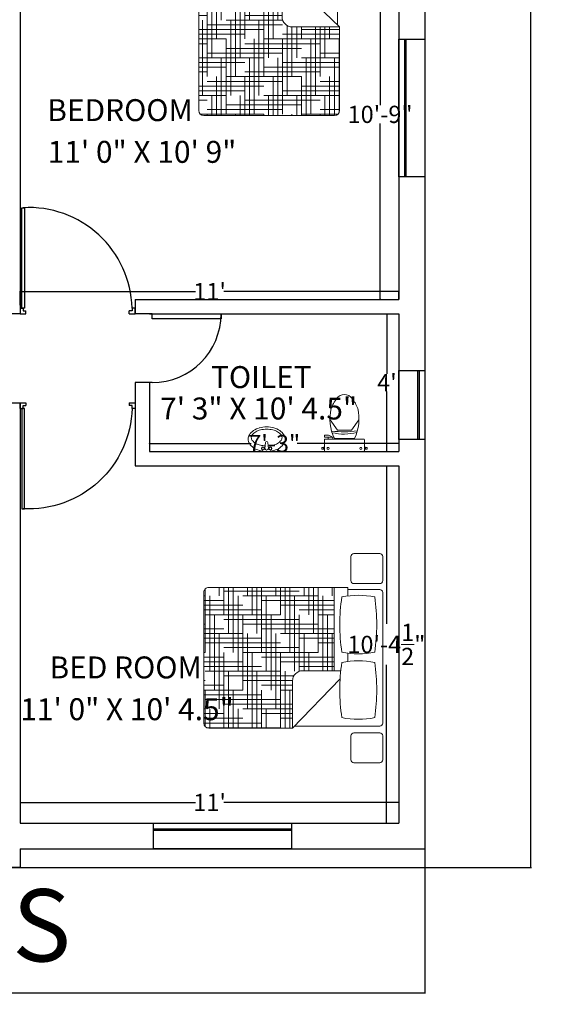
# Model space of a CAD drawing. Units: inches. Extents: x -113 to 5399, y -1393 to 3302.
# Tile 14 of 40: x 1896 to 2086, y 82 to 426. Entities that reach past the tile are written whole.
import ezdxf

# ---------------------------------------------------------------- set-up
doc = ezdxf.new("R2010")
doc.units = ezdxf.units.IN
doc.header["$MEASUREMENT"] = 0
for name, color, linetype, lineweight in [('A-ANNO-DIMS', 254, 'Continuous', 18), ('A-ANNO-TEXT', 7, 'Continuous', 25), ('A-AREA-IDEN', 4, 'Continuous', 18), ('A-FLOR-FIXT', 8, 'Continuous', 18), ('doors', 2, 'Continuous', 25), ('furniture', 131, 'Continuous', 18), ('walls', 1, 'Continuous', 25), ('windows', 3, 'Continuous', 25)]:
    doc.layers.add(name, color=color, linetype=linetype, lineweight=lineweight)
doc.layers.add('A-GLAZ-PATT', color=85, linetype='Continuous', lineweight=13, true_color=0x58ba48)
doc.styles.get("Standard").update_dxf_attribs({"font": 'arial.ttf'})
doc.dimstyles.get("Standard").update_dxf_attribs({"dimtxt": 6, "dimasz": 0.18, "dimexe": 0.18, "dimexo": 0.0625, "dimgap": 0.09, "dimtad": 0, "dimtih": 1, "dimtoh": 1, "dimdec": 1, "dimzin": 0, "dimdsep": 46, "dimlunit": 4, "dimtxsty": 'Standard', "dimblk": 'ARCHTICK', "dimcen": 0.09, "dimadec": 0, "dimazin": 0, "dimtfac": 1, "dimtdec": 1, "dimtofl": 0, "dimtmove": 0, "dimatfit": 3, "dimfxl": 1, "dimtolj": 1, "dimtzin": 0, "dimarcsym": 0})

# ---------------------------------------------------------------- blocks, each defined once
blk = doc.blocks.new('*U2')
for p, q in [((0, 0), (0, -6)), ((24, 0), (24, -6))]:
    blk.add_line(p, q)
blk.add_lwpolyline([(0, 0), (0, 24), (1.75, 24), (1.75, 0)], close=True)
blk.add_arc((0, 0), 24, 0, 90)
blk = doc.blocks.new('*X4')
at = {"color": 0}
for p, q in [((4.3594, 18.5625), (4.3594, 18.6457)), ((4.5, 18), (4.5, 18.6457)), ((4.5469, 18.1875), (4.5469, 18.6457)), ((4.5938, 18.375), (4.5938, 18.6457)), ((4.6406, 18.5625), (4.6406, 18.6457)), ((4.7812, 18), (4.7812, 18.6457)), ((4.8281, 18.1875), (4.8281, 18.6457)), ((4.875, 18.375), (4.875, 18.6457)), ((4.9219, 18.5625), (4.9219, 18.6457)), ((5.0625, 18), (5.0625, 18.6457)), ((5.1094, 18.1875), (5.1094, 18.6457)), ((5.1562, 18.375), (5.1562, 18.6457)), ((5.2031, 18.5625), (5.2031, 18.6457)), ((5.3438, 18), (5.3438, 18.6457)), ((5.3906, 18.1875), (5.3906, 18.6457)), ((5.4375, 18.375), (5.4375, 18.6457)), ((5.4844, 18.5625), (5.4844, 18.6457)), ((5.625, 18), (5.625, 18.6287)), ((4.4531, 17.8169), (4.4531, 18.5625)), ((4.5, 18.5625), (5.25, 18.5625)), ((4.6875, 18.6094), (5.4375, 18.6094)), ((4.7344, 17.8125), (4.7344, 18.5625)), ((5.0156, 17.8125), (5.0156, 18.5625)), ((5.2969, 17.8125), (5.2969, 18.5625)), ((5.5781, 17.8125), (5.5781, 18.5625)), ((5.625, 18.5625), (5.6375, 18.5625)), ((4.3395, 18.5156), (5.0625, 18.5156)), ((4.3395, 18.4688), (4.875, 18.4688)), ((5.25, 18.4688), (5.6375, 18.4688)), ((5.4375, 18.5156), (5.6375, 18.5156)), ((4.3395, 18.4219), (4.6875, 18.4219)), ((4.3395, 18.375), (4.5, 18.375)), ((4.4062, 17.8169), (4.4062, 18.375)), ((4.6875, 17.8114), (4.6875, 18.375)), ((4.6875, 18.3281), (5.4375, 18.3281)), ((4.875, 18.375), (5.625, 18.375)), ((4.9688, 17.625), (4.9688, 18.375)), ((5.0625, 18.4219), (5.6375, 18.4219)), ((5.25, 17.625), (5.25, 18.375)), ((5.5312, 17.625), (5.5312, 18.375)), ((4.3395, 18.2344), (5.0625, 18.2344)), ((4.5, 18.2812), (5.25, 18.2812)), ((5.4375, 18.2344), (5.6375, 18.2344)), ((5.625, 18.2812), (5.6375, 18.2812)), ((4.3395, 18.1875), (4.875, 18.1875)), ((4.3395, 18.1406), (4.6875, 18.1406)), ((4.3594, 17.8169), (4.3594, 18.1875)), ((4.6406, 17.8169), (4.6406, 18.1875)), ((4.9219, 17.4375), (4.9219, 18.1875)), ((5.0625, 18.1406), (5.6375, 18.1406)), ((5.2031, 17.4375), (5.2031, 18.1875)), ((5.25, 18.1875), (5.6375, 18.1875)), ((5.4844, 17.4375), (5.4844, 18.1875)), ((4.3395, 18.0938), (4.5, 18.0938)), ((4.6875, 18.0469), (5.4375, 18.0469)), ((4.875, 18.0938), (5.625, 18.0938)), ((4.3395, 17.9531), (5.0625, 17.9531)), ((4.5, 18), (5.25, 18)), ((4.5938, 17.8169), (4.5938, 18)), ((4.875, 17.25), (4.875, 18)), ((5.1562, 17.25), (5.1562, 18)), ((5.4375, 17.25), (5.4375, 18)), ((5.4375, 17.9531), (5.6375, 17.9531)), ((5.625, 18), (5.6375, 18)), ((4.3395, 17.9062), (4.875, 17.9062)), ((4.3395, 17.8594), (4.6875, 17.8594)), ((5.0625, 17.8594), (5.6375, 17.8594)), ((5.25, 17.9062), (5.6375, 17.9062)), ((4.7421, 17.7656), (5.4375, 17.7656)), ((4.8281, 17.2457), (4.8281, 17.8125)), ((4.875, 17.8125), (5.625, 17.8125)), ((5.1094, 17.2457), (5.1094, 17.8125)), ((5.3906, 17.2457), (5.3906, 17.8125)), ((4.7548, 17.7188), (5.25, 17.7188)), ((4.7548, 17.6719), (5.0625, 17.6719)), ((5.4375, 17.6719), (5.6375, 17.6719)), ((5.625, 17.7188), (5.6375, 17.7188)), ((4.7548, 17.625), (4.875, 17.625)), ((4.7812, 17.2457), (4.7812, 17.625)), ((5.0625, 17.2457), (5.0625, 17.625)), ((5.0625, 17.5781), (5.6375, 17.5781)), ((5.25, 17.625), (5.6375, 17.625)), ((5.3438, 17.2457), (5.3438, 17.625)), ((5.625, 17.2627), (5.625, 17.625)), ((4.7548, 17.4844), (5.4375, 17.4844)), ((4.875, 17.5312), (5.625, 17.5312)), ((4.7548, 17.4375), (5.25, 17.4375)), ((4.7548, 17.3906), (5.0625, 17.3906)), ((5.0156, 17.2457), (5.0156, 17.4375)), ((5.2969, 17.2457), (5.2969, 17.4375)), ((5.4375, 17.3906), (5.6375, 17.3906)), ((5.5781, 17.2457), (5.5781, 17.4375)), ((5.625, 17.4375), (5.6375, 17.4375)), ((4.7548, 17.3438), (4.875, 17.3438)), ((4.875, 17.25), (5.6077, 17.25)), ((4.9688, 17.2457), (4.9688, 17.25)), ((5.0625, 17.2969), (5.6375, 17.2969)), ((5.25, 17.3438), (5.6375, 17.3438)), ((5.25, 17.2457), (5.25, 17.25)), ((5.5312, 17.2457), (5.5312, 17.25))]:
    blk.add_line(p, q, dxfattribs=at)
blk = doc.blocks.new('MAT-P01')
for p, q in [((-0.0213, 0.8164), (-0.0213, 0.5605)), ((0.0087, 0.8464), (0.2471, 0.8464)), ((0.2771, 0.8164), (0.2771, 0.5605)), ((0.3437, 0.8164), (0.3437, -0.0316)), ((0.3737, 0.8464), (1.6737, 0.8464)), ((1.7037, 0.8164), (1.7037, 0.5005)), ((1.7622, 0.8164), (1.7622, 0.5605)), ((1.7922, 0.8464), (2.0306, 0.8464)), ((2.0606, 0.8164), (2.0606, 0.5605)), ((0.0087, 0.5305), (0.2471, 0.5305)), ((0.9879, 0.5005), (1.0693, 0.5005)), ((1.6393, 0.5005), (1.7237, 0.5005)), ((1.7237, 0.5005), (1.7237, -0.8836)), ((1.7922, 0.5305), (2.0306, 0.5305)), ((0.8146, 0.423), (0.3237, -0.0509)), ((0.8949, 0.4293), (0.8949, 0.0491)), ((0.8949, 0.3643), (1.7237, 0.3643)), ((0.8949, 0.3643), (0.8949, 0.0491)), ((0.8949, 0.3643), (1.7237, 0.3643)), ((1.7237, 0.3643), (1.7237, -0.8836)), ((0.3237, -0.0509), (0.7949, -0.0509)), ((0.3237, -0.0509), (0.3237, -0.8836)), ((0.3737, -0.9336), (1.6737, -0.9336))]:
    blk.add_line(p, q)
for centre, radius, start, end in [((0.0087, 0.8164), 0.03, 90, 180), ((0.2471, 0.8164), 0.03, 0, 90), ((0.3737, 0.8164), 0.03, 90, 180), ((0.7029, -1.1436), 1.9306, 81.81622, 98.18378), ((1.3543, -1.1436), 1.9306, 81.81622, 98.18378), ((1.6737, 0.8164), 0.03, 0, 90), ((1.7922, 0.8164), 0.03, 90, 180), ((2.0306, 0.8164), 0.03, 0, 90), ((1.2251, 0.6034), 0.8138, 168.37298, 191.62702), ((0.1806, 0.6034), 0.8138, 348.37298, 11.62702), ((1.8766, 0.6034), 0.8138, 168.37298, 191.62702), ((0.8321, 0.6034), 0.8138, 348.37298, 11.62702), ((0.0087, 0.5605), 0.03, 180, 270), ((0.2471, 0.5605), 0.03, 270, 0), ((1.7922, 0.5605), 0.03, 180, 270), ((2.0306, 0.5605), 0.03, 270, 0), ((0.7029, 2.3504), 1.9306, 261.81622, 278.18378), ((1.3543, 2.3504), 1.9306, 261.81622, 278.18378), ((0.7949, 0.0491), 0.1, 270, 0), ((0.3737, -0.8836), 0.05, 180, 270), ((1.6737, -0.8836), 0.05, 270, 0)]:
    blk.add_arc(centre, radius, start, end)
at = {"rotation": 270}
blk.add_blockref('*X4', (-16.9221, 4.7038), dxfattribs=at)
blk = doc.blocks.new('toilet-3')
at = {"color": 0, "linetype": 'ByBlock'}
for p, q in [((-0.281, -0.05), (-0.281, -0.069)), ((-0.281, -0.05), (-0.261, -0.05)), ((-0.281, -0.069), (-0.261, -0.069)), ((-0.261, -0.047), (-0.261, -0.072)), ((-0.261, -0.047), (-0.251, -0.047)), ((-0.261, -0.072), (-0.251, -0.072)), ((-0.251, -0.047), (-0.251, -0.072)), ((-0.25, -0.03), (-0.25, -0.165)), ((0.24, -0.02), (-0.24, -0.02)), ((0.25, -0.03), (0.25, -0.165)), ((0.261, -0.047), (0.251, -0.047)), ((0.251, -0.047), (0.251, -0.072)), ((0.261, -0.072), (0.251, -0.072)), ((0.261, -0.047), (0.261, -0.072)), ((0.281, -0.05), (0.261, -0.05)), ((0.281, -0.069), (0.261, -0.069)), ((0.281, -0.05), (0.281, -0.069)), ((-0.144, -0.2), (-0.25, -0.2)), ((-0.25, -0.2), (-0.25, -0.222)), ((-0.198, -0.222), (-0.25, -0.222)), ((0.24, -0.175), (-0.24, -0.175)), ((-0.202, -0.2), (-0.202, -0.175)), ((-0.198, -0.222), (-0.16, -0.207)), ((-0.16, -0.207), (-0.16, -0.2)), ((-0.144, -0.2), (-0.144, -0.175)), ((0.125, -0.182), (-0.125, -0.182)), ((-0.089, -0.287), (-0.18, -0.415)), ((0.089, -0.287), (-0.089, -0.287)), ((0.089, -0.287), (0.18, -0.415))]:
    blk.add_line(p, q, dxfattribs=at)
for centre in [(-0.205, -0.059), (0.205, -0.059)]:
    blk.add_circle(centre, 0.0125, dxfattribs=at)
for centre, radius, start, end in [((-0.24, -0.03), 0.01, 90, 180), ((0.24, -0.03), 0.01, 0, 90), ((-0.24, -0.165), 0.01, 180, 270), ((0.376, -0.424), 0.557, 154.2321, 193.6755), ((-0.005, -0.896), 0.659, 75.9276, 103.0204), ((-0.376, -0.424), 0.557, 346.3245, 25.7679), ((0.24, -0.165), 0.01, 270, 0), ((-0.013, -1.787), 1.521, 83.4552, 95.5271), ((0.262, -0.406), 0.452, 199.2942, 217.2549), ((-0.265, -0.4), 0.457, 322.2382, 340.1051), ((-0.001, -0.609), 0.12, 216.3794, 323.6206)]:
    blk.add_arc(centre, radius, start, end, dxfattribs=at)
blk = doc.blocks.new('wash-6')
at = {"color": 0, "linetype": 'ByBlock'}
for p, q in [((-0.036, -0.063), (-0.021, -0.18)), ((0.036, -0.063), (0.021, -0.18))]:
    blk.add_line(p, q, dxfattribs=at)
for centre, radius in [((-0.075, -0.062), 0.0325), ((-0.075, -0.062), 0.0263), ((0.075, -0.062), 0.0325), ((0.075, -0.062), 0.0263)]:
    blk.add_circle(centre, radius, dxfattribs=at)
for centre, radius, start, end in [((0, -0.56), 0.56, 90, 105.4371), ((-0.204, -0.25), 0.17, 148.1465, 180), ((-0.107, -0.311), 0.285, 123.6901, 148.1465), ((-0.114, -0.361), 0.225, 118.369, 142.5096), ((-0.042, -0.407), 0.401, 105.4371, 123.6901), ((-0.045, -0.488), 0.37, 102.6081, 118.369), ((0, -0.69), 0.576, 92.9466, 102.6081), ((0, -0.063), 0.0361, 0, 180), ((0, -0.18), 0.0215, 180, 0), ((0, -0.56), 0.56, 74.5629, 90), ((0, -0.69), 0.576, 77.3919, 87.0534), ((0.045, -0.488), 0.37, 61.631, 77.3919), ((0.042, -0.407), 0.401, 56.3099, 74.5629), ((0.114, -0.361), 0.225, 37.4904, 61.631), ((0.107, -0.311), 0.285, 31.8535, 56.3099), ((0.204, -0.25), 0.17, 0, 31.8535), ((-0.204, -0.25), 0.17, 180, 211.8535), ((-0.107, -0.189), 0.285, 211.8535, 236.3099), ((-0.217, -0.282), 0.0954, 142.5096, 180), ((-0.217, -0.282), 0.0954, 180, 217.4904), ((-0.114, -0.203), 0.225, 217.4904, 241.631), ((0.114, -0.203), 0.225, 298.369, 322.5096), ((0.107, -0.189), 0.285, 303.6901, 328.1465), ((0.217, -0.282), 0.0954, 0, 37.4904), ((0.217, -0.282), 0.0954, 322.5096, 0), ((0.204, -0.25), 0.17, 328.1465, 0), ((-0.042, -0.092), 0.401, 236.3099, 254.5629), ((-0.045, -0.076), 0.37, 241.631, 257.3919), ((0, 0.06), 0.56, 254.5629, 270), ((0, 0.125), 0.576, 257.3919, 270), ((0, 0.125), 0.576, 270, 282.6081), ((0, 0.06), 0.56, 270, 285.4371), ((0.045, -0.076), 0.37, 282.6081, 298.369), ((0.042, -0.092), 0.401, 285.4371, 303.6901)]:
    blk.add_arc(centre, radius, start, end, dxfattribs=at)
blk = doc.blocks.new('_ArchTick')
at = {"color": 0, "linetype": 'ByBlock', "const_width": 0.15}
blk.add_lwpolyline([(-0.5, -0.5), (0.5, 0.5)], dxfattribs=at)
blk = doc.blocks.new('*D59')
at = {"layer": 'A-ANNO-DIMS', "color": 0, "lineweight": -2, "transparency": 16777216}
for p, q in [((1604.26, 136.47), (1604.26, 86.09)), ((2037.26, 136.47), (2037.26, 86.09)), ((1604.26, 86.27), (1810.37, 86.27)), ((2037.26, 86.27), (1831.16, 86.27))]:
    blk.add_line(p, q, dxfattribs=at)
at = {"layer": 'Defpoints', "color": 0, "transparency": 16777216}
for p in [(1604.26, 136.53), (2037.26, 136.53), (2037.26, 86.27)]:
    blk.add_point(p, dxfattribs=at)
at = {"layer": 'A-ANNO-DIMS', "color": 0, "lineweight": -2, "transparency": 16777216, "xscale": 0.18, "yscale": 0.18, "zscale": 0.18, "rotation": 180}
blk.add_blockref('_ArchTick', (1604.26, 86.27), dxfattribs=at)
at = {"layer": 'A-ANNO-DIMS', "color": 0, "lineweight": -2, "transparency": 16777216, "xscale": 0.18, "yscale": 0.18, "zscale": 0.18}
blk.add_blockref('_ArchTick', (2037.26, 86.27), dxfattribs=at)
at = {"layer": 'A-ANNO-DIMS', "color": 0, "transparency": 16777216, "insert": (1820.76, 86.27), "char_height": 6, "attachment_point": 5}
blk.add_mtext('\\A1;36\'-1"', dxfattribs=at)
blk = doc.blocks.new('*D63')
at = {"layer": 'A-ANNO-DIMS', "color": 0, "lineweight": -2, "transparency": 16777216}
for p, q in [((2021.95, 457.03), (2021.49, 457.03)), ((2021.67, 457.03), (2021.67, 395.69)), ((2021.67, 328.03), (2021.67, 389.38)), ((2021.95, 328.03), (2021.49, 328.03))]:
    blk.add_line(p, q, dxfattribs=at)
at = {"layer": 'Defpoints', "color": 0, "transparency": 16777216}
for p in [(2022.01, 457.03), (2021.67, 328.03), (2022.01, 328.03)]:
    blk.add_point(p, dxfattribs=at)
at = {"layer": 'A-ANNO-DIMS', "color": 0, "lineweight": -2, "transparency": 16777216, "xscale": 0.18, "yscale": 0.18, "zscale": 0.18}
for p, rotation in [((2021.67, 457.03), 90), ((2021.67, 328.03), 270)]:
    blk.add_blockref('_ArchTick', p, dxfattribs=dict(at, rotation=rotation))
at = {"layer": 'A-ANNO-DIMS', "color": 0, "transparency": 16777216, "insert": (2021.67, 392.53), "char_height": 6, "attachment_point": 5}
blk.add_mtext('\\A1;10\'-9"', dxfattribs=at)
blk = doc.blocks.new('*D64')
at = {"layer": 'A-ANNO-DIMS', "color": 0, "lineweight": -2, "transparency": 16777216}
for p, q in [((1896.26, 326.08), (1896.26, 330.94)), ((1896.26, 330.76), (1957.36, 330.76)), ((2028.26, 330.76), (1967.16, 330.76)), ((2028.26, 328.09), (2028.26, 330.94))]:
    blk.add_line(p, q, dxfattribs=at)
at = {"layer": 'Defpoints', "color": 0, "transparency": 16777216}
for p in [(2028.26, 330.76), (2028.26, 328.03), (1896.26, 326.02)]:
    blk.add_point(p, dxfattribs=at)
at = {"layer": 'A-ANNO-DIMS', "color": 0, "lineweight": -2, "transparency": 16777216, "xscale": 0.18, "yscale": 0.18, "zscale": 0.18, "rotation": 180}
blk.add_blockref('_ArchTick', (1896.26, 330.76), dxfattribs=at)
at = {"layer": 'A-ANNO-DIMS', "color": 0, "lineweight": -2, "transparency": 16777216, "xscale": 0.18, "yscale": 0.18, "zscale": 0.18}
blk.add_blockref('_ArchTick', (2028.26, 330.76), dxfattribs=at)
at = {"layer": 'A-ANNO-DIMS', "color": 0, "transparency": 16777216, "insert": (1962.26, 330.76), "char_height": 6, "attachment_point": 5}
blk.add_mtext("\\A1;11'", dxfattribs=at)
blk = doc.blocks.new('*D65')
at = {"layer": 'A-ANNO-DIMS', "color": 0, "lineweight": -2, "transparency": 16777216}
for p, q in [((2023.85, 323.03), (2024.23, 323.03)), ((2024.05, 323.03), (2024.05, 302.12)), ((2024.05, 275.03), (2024.05, 295.94)), ((2023.85, 275.03), (2024.23, 275.03))]:
    blk.add_line(p, q, dxfattribs=at)
at = {"layer": 'Defpoints', "color": 0, "transparency": 16777216}
for p in [(2023.79, 323.03), (2023.79, 275.03), (2024.05, 275.03)]:
    blk.add_point(p, dxfattribs=at)
at = {"layer": 'A-ANNO-DIMS', "color": 0, "lineweight": -2, "transparency": 16777216, "xscale": 0.18, "yscale": 0.18, "zscale": 0.18}
for p, rotation in [((2024.05, 323.03), 90), ((2024.05, 275.03), 270)]:
    blk.add_blockref('_ArchTick', p, dxfattribs=dict(at, rotation=rotation))
at = {"layer": 'A-ANNO-DIMS', "color": 0, "transparency": 16777216, "insert": (2024.05, 299.03), "char_height": 6, "attachment_point": 5}
blk.add_mtext("\\A1;4'", dxfattribs=at)
blk = doc.blocks.new('*D66')
at = {"layer": 'A-ANNO-DIMS', "color": 0, "lineweight": -2, "transparency": 16777216}
for p, q in [((1941.26, 277.84), (1941.26, 277.96)), ((1941.26, 277.78), (1976.72, 277.78)), ((2028.26, 277.78), (1992.8, 277.78)), ((2028.26, 277.84), (2028.26, 277.96))]:
    blk.add_line(p, q, dxfattribs=at)
at = {"layer": 'Defpoints', "color": 0, "transparency": 16777216}
for p in [(1941.26, 277.78), (2028.26, 277.78), (2028.26, 277.78)]:
    blk.add_point(p, dxfattribs=at)
at = {"layer": 'A-ANNO-DIMS', "color": 0, "lineweight": -2, "transparency": 16777216, "xscale": 0.18, "yscale": 0.18, "zscale": 0.18, "rotation": 180}
blk.add_blockref('_ArchTick', (1941.26, 277.78), dxfattribs=at)
at = {"layer": 'A-ANNO-DIMS', "color": 0, "lineweight": -2, "transparency": 16777216, "xscale": 0.18, "yscale": 0.18, "zscale": 0.18}
blk.add_blockref('_ArchTick', (2028.26, 277.78), dxfattribs=at)
at = {"layer": 'A-ANNO-DIMS', "color": 0, "transparency": 16777216, "insert": (1984.76, 277.78), "char_height": 6, "attachment_point": 5}
blk.add_mtext('\\A1;7\'-3"', dxfattribs=at)
blk = doc.blocks.new('*D79')
at = {"layer": 'A-ANNO-DIMS', "color": 0, "lineweight": -2, "transparency": 16777216}
for p, q in [((2022.75, 270.03), (2024.05, 270.03)), ((2023.87, 270.03), (2023.87, 214.95)), ((2023.87, 145.53), (2023.87, 200.62)), ((2022.75, 145.53), (2024.05, 145.53))]:
    blk.add_line(p, q, dxfattribs=at)
at = {"layer": 'Defpoints', "color": 0, "transparency": 16777216}
for p in [(2022.68, 270.03), (2022.68, 145.53), (2023.87, 145.53)]:
    blk.add_point(p, dxfattribs=at)
at = {"layer": 'A-ANNO-DIMS', "color": 0, "lineweight": -2, "transparency": 16777216, "xscale": 0.18, "yscale": 0.18, "zscale": 0.18}
for p, rotation in [((2023.87, 270.03), 90), ((2023.87, 145.53), 270)]:
    blk.add_blockref('_ArchTick', p, dxfattribs=dict(at, rotation=rotation))
at = {"layer": 'A-ANNO-DIMS', "color": 0, "transparency": 16777216, "insert": (2023.87, 207.78), "char_height": 6, "attachment_point": 5}
blk.add_mtext('\\A1;10\'-4{\\H1x;\\S1/2;}"', dxfattribs=at)
blk = doc.blocks.new('*D80')
at = {"layer": 'A-ANNO-DIMS', "color": 0, "lineweight": -2, "transparency": 16777216}
for p, q in [((1896.26, 152.81), (1896.26, 152.53)), ((1896.26, 152.71), (1957.36, 152.71)), ((2028.26, 152.71), (1967.16, 152.71)), ((2028.26, 152.81), (2028.26, 152.53))]:
    blk.add_line(p, q, dxfattribs=at)
at = {"layer": 'Defpoints', "color": 0, "transparency": 16777216}
for p in [(1896.26, 152.87), (2028.26, 152.87), (2028.26, 152.71)]:
    blk.add_point(p, dxfattribs=at)
at = {"layer": 'A-ANNO-DIMS', "color": 0, "lineweight": -2, "transparency": 16777216, "xscale": 0.18, "yscale": 0.18, "zscale": 0.18, "rotation": 180}
blk.add_blockref('_ArchTick', (1896.26, 152.71), dxfattribs=at)
at = {"layer": 'A-ANNO-DIMS', "color": 0, "lineweight": -2, "transparency": 16777216, "xscale": 0.18, "yscale": 0.18, "zscale": 0.18}
blk.add_blockref('_ArchTick', (2028.26, 152.71), dxfattribs=at)
at = {"layer": 'A-ANNO-DIMS', "color": 0, "transparency": 16777216, "insert": (1962.26, 152.71), "char_height": 6, "attachment_point": 5}
blk.add_mtext("\\A1;11'", dxfattribs=at)
blk = doc.blocks.new('WIN-PLAN-48IN')
h = blk.add_hatch(color=256)
h.dxf.hatch_style = 1
h.paths.add_polyline_path([(48, 2.5), (0, 2.5), (0, 2), (48, 2)])
for p, q in [((0, 9), (48, 9)), ((0, 0), (0, 9)), ((48, 9), (48, 0)), ((48, 2.5), (0, 2.5)), ((48, 2), (0, 2)), ((48, 0), (0, 0))]:
    blk.add_line(p, q)
blk = doc.blocks.new('DOOR-SINGLE-36IN-PLAN')
for p, q in [((0.5, 2), (0.5, 36.98)), ((0.5, 36.98), (1.5, 36.98)), ((1.5, 36.98), (1.5, 2)), ((0, 2), (0, 0)), ((0, 2), (1.04, 2)), ((1.5, 2), (0.5, 2)), ((1.04, 2), (1.04, 0.98)), ((1.04, 0.98), (2, 0.98)), ((2, 0), (2, 0.98)), ((38.96, 0.98), (38, 0.98)), ((38, 0), (38, 0.98)), ((40, 2), (38.96, 2)), ((38.96, 2), (38.96, 0.98)), ((40, 0), (40, 2)), ((0, 0), (2, 0)), ((0, 0), (2, 0)), ((38, 0), (40, 0))]:
    blk.add_line(p, q)
blk.add_arc((2.94, 0.99), 36.04, 1.6003, 93.0893)
blk = doc.blocks.new('*D209')
at = {"layer": 'A-ANNO-DIMS', "color": 0, "lineweight": -2, "transparency": 16777216}
for p, q in [((1754.32, 798.03), (2074.39, 798.03)), ((2074.21, 798.03), (2074.21, 467.19)), ((2074.21, 130.03), (2074.21, 460.88)), ((1754.32, 130.03), (2074.39, 130.03))]:
    blk.add_line(p, q, dxfattribs=at)
at = {"layer": 'Defpoints', "color": 0, "transparency": 16777216}
for p in [(1754.26, 798.03), (2074.21, 798.03), (1754.26, 130.03)]:
    blk.add_point(p, dxfattribs=at)
at = {"layer": 'A-ANNO-DIMS', "color": 0, "lineweight": -2, "transparency": 16777216, "xscale": 0.18, "yscale": 0.18, "zscale": 0.18}
for p, rotation in [((2074.21, 798.03), 90), ((2074.21, 130.03), 270)]:
    blk.add_blockref('_ArchTick', p, dxfattribs=dict(at, rotation=rotation))
at = {"layer": 'A-ANNO-DIMS', "color": 0, "transparency": 16777216, "insert": (2074.21, 464.03), "char_height": 6, "attachment_point": 5}
blk.add_mtext('\\A1;55\'-8"', dxfattribs=at)

msp = doc.modelspace()

# ---------------------------------------------------------------- hatches: boundary and pattern name
at = {"layer": 'A-GLAZ-PATT'}
h = msp.add_hatch(color=256, dxfattribs=at)
h.dxf.hatch_style = 1
h.paths.add_polyline_path([(2034.76, 303.22), (2034.76, 279.22), (2035.26, 279.22), (2035.26, 303.22)])

# ---------------------------------------------------------------- linework, layer by layer
at = {"layer": 'walls'}
for p, q in [((2037.26, 786.53), (2037.26, 136.53)), ((1896.26, 457.03), (1896.26, 325.03)), ((2028.26, 457.03), (2028.26, 332.53)), ((2028.26, 332.53), (2028.26, 328.03)), ((1936.26, 328.03), (1936.26, 323.03)), ((1936.26, 328.03), (2028.26, 328.03)), ((1896.26, 323.03), (1891.26, 323.03)), ((1941.26, 323.03), (1936.26, 323.03)), ((1941.26, 323.03), (2028.26, 323.03)), ((2028.26, 323.03), (2028.26, 275.03)), ((1936.26, 299.03), (1936.26, 270.03)), ((1941.26, 299.03), (1936.26, 299.03)), ((1941.26, 299.03), (1941.26, 275.03)), ((1891.26, 292.03), (1896.26, 292.03)), ((1896.26, 292.03), (1896.26, 145.53)), ((1941.26, 275.03), (2028.26, 275.03)), ((1936.26, 270.03), (2028.26, 270.03)), ((2028.26, 270.03), (2028.26, 145.53)), ((1896.26, 145.53), (2028.26, 145.53)), ((1896.26, 136.53), (2037.26, 136.53)), ((1896.26, 136.53), (1896.26, 130.03)), ((1896.26, 130.03), (1891.26, 130.03))]:
    msp.add_line(p, q, dxfattribs=at)
at = {"layer": 'windows'}
for p, q in [((2028.26, 279.22), (2028.26, 303.22)), ((2028.26, 303.22), (2037.26, 303.22)), ((2034.76, 303.22), (2034.76, 279.22)), ((2035.26, 303.22), (2035.26, 279.22)), ((2037.26, 303.22), (2037.26, 279.22)), ((2037.26, 279.22), (2028.26, 279.22))]:
    msp.add_line(p, q, dxfattribs=at)

# ---------------------------------------------------------------- block references
at = {"layer": 'A-FLOR-FIXT', "rotation": 180}
for name, p, xscale, yscale, zscale in [('toilet-3', (2009.26, 274.47), -27.95492935005888, 27.95492935005888, 27.95492935005888), ('wash-6', (1982.14, 275.03), -17.16666334294967, 17.16666334294967, 17.16666334294967)]:
    msp.add_blockref(name, p, dxfattribs=dict(at, xscale=xscale, yscale=yscale, zscale=zscale))
at = {"layer": 'doors'}
msp.add_blockref('DOOR-SINGLE-36IN-PLAN', (1896.26, 323.03), dxfattribs=at)
at = {"layer": 'doors', "rotation": 270}
msp.add_blockref('*U2', (1942.26, 323.03), dxfattribs=at)
at = {"layer": 'doors', "extrusion": (0, 0, -1), "zscale": -1, "rotation": 180}
msp.add_blockref('DOOR-SINGLE-36IN-PLAN', (-1896.26, 292.03), dxfattribs=at)
at = {"layer": 'furniture', "xscale": -35.02364872074636, "yscale": 35.02364872074636, "zscale": 35.02364872074636}
msp.add_blockref('MAT-P01', (2018.86, 424.81), dxfattribs=at)
at = {"layer": 'furniture', "xscale": -35.02364872074636, "yscale": 35.02364872074636, "zscale": 35.02364872074636, "rotation": 270}
msp.add_blockref('MAT-P01', (1992.94, 167.26), dxfattribs=at)
at = {"layer": 'windows'}
for p, rotation in [((2028.26, 418.78), 269.9999999999994), ((1990.76, 145.53), 180)]:
    msp.add_blockref('WIN-PLAN-48IN', p, dxfattribs=dict(at, rotation=rotation))

# ---------------------------------------------------------------- texts
at = {"layer": 'A-ANNO-TEXT'}
msp.add_text('1,2,3,4 FLOORS', height=25.17, dxfattribs=at).set_placement((1670.55, 97.29))
at = {"layer": 'A-AREA-IDEN'}
for s, height, p in [('BEDROOM', 7.647, (1905.66, 390.18)), ('11\' 0" X 10\' 9"', 7.6473, (1905.83, 375.64)), ('TOILET', 7.647, (1962.74, 297.13)), ('7\' 3" X 10\' 4.5"', 7.6473, (1945.02, 286.18)), ('BED ROOM', 7.647, (1906.45, 195.93)), ('11\' 0" X 10\' 4.5"', 7.6473, (1896.26, 181.37))]:
    msp.add_text(s, height=height, dxfattribs=at).set_placement(p)

# ---------------------------------------------------------------- dimensions: what is measured, and where the dimension line sits
at = {"layer": 'A-ANNO-DIMS'}
for base, p1, p2, override, picture, middle in [((2074.21, 798.03), (1754.26, 130.03), (1754.26, 798.03), {"dimdec": 1, "dimlfac": 1, "dimrnd": 0, "dimzin": 1, "dimdsep": 46, "dimlunit": 4, "dimfrac": 2}, '*D209', (2074.21, 464.03)), ((2021.67, 328.03), (2022.01, 457.03), (2022.01, 328.03), {"dimclrd": 0, "dimclre": 0, "dimclrt": 0}, '*D63', (2021.67, 392.53)), ((2024.05, 275.03), (2023.79, 323.03), (2023.79, 275.03), {"dimclrd": 0, "dimclre": 0, "dimclrt": 0}, '*D65', (2024.05, 299.03)), ((2023.87, 145.53), (2022.68, 270.03), (2022.68, 145.53), {"dimclrd": 0, "dimclre": 0, "dimclrt": 0}, '*D79', (2023.87, 207.78))]:
    dim = msp.add_linear_dim(base=base, p1=p1, p2=p2, angle=90, dimstyle='Standard', override=override, dxfattribs=at)
    dim.commit()
    dim.dimension.update_dxf_attribs({"geometry": picture, "text_midpoint": middle})
for base, p1, p2, picture, middle in [((2028.26, 330.76), (1896.26, 326.02), (2028.26, 328.03), '*D64', (1962.26, 330.76)), ((2028.26, 277.78), (1941.26, 277.78), (2028.26, 277.78), '*D66', (1984.76, 277.78)), ((2028.26, 152.71), (1896.26, 152.87), (2028.26, 152.87), '*D80', (1962.26, 152.71)), ((2037.26, 86.27), (1604.26, 136.53), (2037.26, 136.53), '*D59', (1820.76, 86.27))]:
    dim = msp.add_linear_dim(base=base, p1=p1, p2=p2, dimstyle='Standard', override={"dimclrd": 0, "dimclre": 0, "dimclrt": 0}, dxfattribs=at)
    dim.commit()
    dim.dimension.update_dxf_attribs({"geometry": picture, "text_midpoint": middle})

doc.saveas('drawing.dxf')
